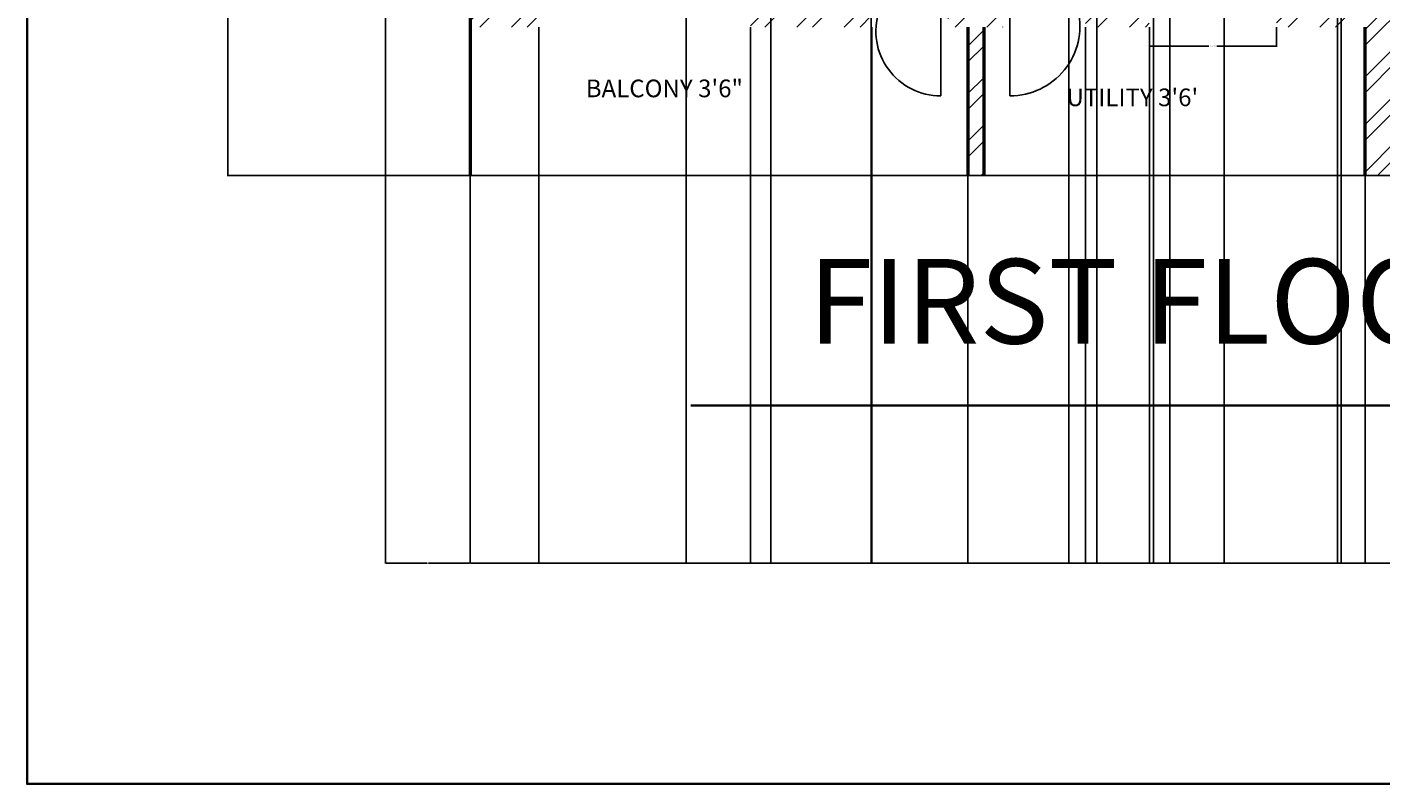
# Model space of a CAD drawing. Units: inches. Extents: x 1980 to 2738, y 1471 to 2568.
# Tile 1 of 22: x 1980 to 2363, y 1471 to 1686. Entities that reach past the tile are written whole.
import ezdxf

# ---------------------------------------------------------------- set-up
doc = ezdxf.new("R2010")
doc.units = ezdxf.units.IN
for name, color, linetype, lineweight in [('A-ANNO-DIMS', 2, 'Continuous', 18), ('A-ANNO-TTLB', 7, 'Continuous', 35), ('A-AREA-IDEN', 7, 'Continuous', 18), ('A-DOOR', 31, 'Continuous', 25), ('A-FLOR-BALC', 7, 'Continuous', 25), ('A-WALL', 7, 'Continuous', 50)]:
    doc.layers.add(name, color=color, linetype=linetype, lineweight=lineweight)
doc.layers.add('A-WALL-PATT', color=9, linetype='Continuous', lineweight=13, true_color=0xd19cc7)
doc.styles.get("Standard").update_dxf_attribs({"font": 'arial.ttf'})
doc.dimstyles.get("Standard").update_dxf_attribs({"dimtxt": 0.18, "dimasz": 0.18, "dimexe": 0.18, "dimexo": 0.0625, "dimgap": 0.09, "dimtad": 0, "dimtih": 1, "dimtoh": 1, "dimdec": 4, "dimzin": 0, "dimdsep": 46, "dimtxsty": 'Standard', "dimcen": 0.09, "dimadec": 0, "dimazin": 0, "dimtfac": 1, "dimtdec": 4, "dimtofl": 0, "dimtmove": 0, "dimatfit": 3, "dimfxl": 1, "dimtolj": 1, "dimtzin": 0, "dimarcsym": 0})

# ---------------------------------------------------------------- blocks, each defined once
blk = doc.blocks.new('*D31')
at = {"layer": 'A-ANNO-DIMS', "color": 0, "lineweight": -2, "transparency": 16777216}
for p, q in [((2297.48, 1685.64), (2297.48, 1680.13)), ((2333.48, 1685.64), (2333.48, 1680.13)), ((2297.66, 1680.31), (2314.36, 1680.31)), ((2333.3, 1680.31), (2316.59, 1680.31))]:
    blk.add_line(p, q, dxfattribs=at)
at = {"layer": 'A-ANNO-DIMS', "color": 0, "transparency": 16777216}
for points in [[(2297.66, 1680.34), (2297.66, 1680.28), (2297.48, 1680.31)], [(2333.3, 1680.34), (2333.3, 1680.28), (2333.48, 1680.31)]]:
    blk.add_solid(points, dxfattribs=at)
at = {"layer": 'Defpoints', "color": 0, "transparency": 16777216}
for p in [(2297.48, 1685.71), (2333.48, 1685.71), (2333.48, 1680.31)]:
    blk.add_point(p, dxfattribs=at)
at = {"layer": 'A-ANNO-DIMS', "color": 0, "transparency": 16777216, "insert": (2315.48, 1680.31), "char_height": 0.18, "attachment_point": 5}
blk.add_mtext('\\A1;WINDOW 36 TYP.', dxfattribs=at)
blk = doc.blocks.new('*D36')
at = {"layer": 'A-ANNO-DIMS', "color": 0, "lineweight": -2, "transparency": 16777216}
for p, q in [((2105.02, 2462.71), (2036.25, 2462.71)), ((2036.43, 2462.53), (2036.43, 2053.39)), ((2036.43, 1643.89), (2036.43, 2053.02)), ((2105.02, 1643.71), (2036.25, 1643.71))]:
    blk.add_line(p, q, dxfattribs=at)
at = {"layer": 'A-ANNO-DIMS', "color": 0, "transparency": 16777216}
for points in [[(2036.4, 2462.53), (2036.46, 2462.53), (2036.43, 2462.71)], [(2036.4, 1643.89), (2036.46, 1643.89), (2036.43, 1643.71)]]:
    blk.add_solid(points, dxfattribs=at)
at = {"layer": 'Defpoints', "color": 0, "transparency": 16777216}
for p in [(2036.43, 2462.71), (2105.08, 2462.71), (2105.08, 1643.71)]:
    blk.add_point(p, dxfattribs=at)
at = {"layer": 'A-ANNO-DIMS', "color": 0, "transparency": 16777216, "insert": (2036.43, 2053.21), "char_height": 0.18, "attachment_point": 5}
blk.add_mtext('\\A1;819', dxfattribs=at)
blk = doc.blocks.new('*D40')
at = {"layer": 'A-ANNO-DIMS', "color": 0, "lineweight": -2, "transparency": 16777216}
for p, q in [((2218.65, 2053.14), (2218.65, 1533.71)), ((2298.65, 2053.14), (2298.65, 1533.71)), ((2218.83, 1533.89), (2258.43, 1533.89)), ((2298.47, 1533.89), (2258.87, 1533.89))]:
    blk.add_line(p, q, dxfattribs=at)
at = {"layer": 'A-ANNO-DIMS', "color": 0, "transparency": 16777216}
for points in [[(2218.83, 1533.92), (2218.83, 1533.86), (2218.65, 1533.89)], [(2298.47, 1533.92), (2298.47, 1533.86), (2298.65, 1533.89)]]:
    blk.add_solid(points, dxfattribs=at)
at = {"layer": 'Defpoints', "color": 0, "transparency": 16777216}
for p in [(2218.65, 2053.21), (2298.65, 2053.21), (2298.65, 1533.89)]:
    blk.add_point(p, dxfattribs=at)
at = {"layer": 'A-ANNO-DIMS', "color": 0, "transparency": 16777216, "insert": (2258.65, 1533.89), "char_height": 0.18, "attachment_point": 5}
blk.add_mtext('\\A1;80', dxfattribs=at)
blk = doc.blocks.new('*D41')
at = {"layer": 'A-ANNO-DIMS', "color": 0, "lineweight": -2, "transparency": 16777216}
for p, q in [((2298.65, 2095.14), (2298.65, 1533.71)), ((2515.4, 2095.14), (2515.4, 1533.71)), ((2298.83, 1533.89), (2406.56, 1533.89)), ((2515.22, 1533.89), (2407.49, 1533.89))]:
    blk.add_line(p, q, dxfattribs=at)
at = {"layer": 'A-ANNO-DIMS', "color": 0, "transparency": 16777216}
for points in [[(2298.83, 1533.92), (2298.83, 1533.86), (2298.65, 1533.89)], [(2515.22, 1533.92), (2515.22, 1533.86), (2515.4, 1533.89)]]:
    blk.add_solid(points, dxfattribs=at)
at = {"layer": 'Defpoints', "color": 0, "transparency": 16777216}
for p in [(2298.65, 2095.21), (2515.4, 2095.21), (2515.4, 1533.89)]:
    blk.add_point(p, dxfattribs=at)
at = {"layer": 'A-ANNO-DIMS', "color": 0, "transparency": 16777216, "insert": (2407.03, 1533.89), "char_height": 0.18, "attachment_point": 5}
blk.add_mtext('\\A1;216.75', dxfattribs=at)
blk = doc.blocks.new('*D42')
at = {"layer": 'A-ANNO-DIMS', "color": 0, "lineweight": -2, "transparency": 16777216}
for p, q in [((2105.08, 1685.64), (2105.08, 1533.71)), ((2124.51, 1685.64), (2124.51, 1533.71)), ((2105.26, 1533.89), (2114.34, 1533.89)), ((2124.33, 1533.89), (2115.25, 1533.89))]:
    blk.add_line(p, q, dxfattribs=at)
at = {"layer": 'A-ANNO-DIMS', "color": 0, "transparency": 16777216}
for points in [[(2105.26, 1533.92), (2105.26, 1533.86), (2105.08, 1533.89)], [(2124.33, 1533.92), (2124.33, 1533.86), (2124.51, 1533.89)]]:
    blk.add_solid(points, dxfattribs=at)
at = {"layer": 'Defpoints', "color": 0, "transparency": 16777216}
for p in [(2105.08, 1685.71), (2124.51, 1685.71), (2124.51, 1533.89)]:
    blk.add_point(p, dxfattribs=at)
at = {"layer": 'A-ANNO-DIMS', "color": 0, "transparency": 16777216, "insert": (2114.8, 1533.89), "char_height": 0.18, "attachment_point": 5}
blk.add_mtext('\\A1;19.427', dxfattribs=at)
blk = doc.blocks.new('*D43')
at = {"layer": 'A-ANNO-DIMS', "color": 0, "lineweight": -2, "transparency": 16777216}
for p, q in [((2184.51, 1685.64), (2184.51, 1533.71)), ((2218.88, 1685.64), (2218.88, 1533.71)), ((2184.69, 1533.89), (2201.3, 1533.89)), ((2218.7, 1533.89), (2202.09, 1533.89))]:
    blk.add_line(p, q, dxfattribs=at)
at = {"layer": 'A-ANNO-DIMS', "color": 0, "transparency": 16777216}
for points in [[(2184.69, 1533.92), (2184.69, 1533.86), (2184.51, 1533.89)], [(2218.7, 1533.92), (2218.7, 1533.86), (2218.88, 1533.89)]]:
    blk.add_solid(points, dxfattribs=at)
at = {"layer": 'Defpoints', "color": 0, "transparency": 16777216}
for p in [(2184.51, 1685.71), (2218.88, 1685.71), (2218.88, 1533.89)]:
    blk.add_point(p, dxfattribs=at)
at = {"layer": 'A-ANNO-DIMS', "color": 0, "transparency": 16777216, "insert": (2201.69, 1533.89), "char_height": 0.18, "attachment_point": 5}
blk.add_mtext('\\A1;34.37', dxfattribs=at)
blk = doc.blocks.new('*D47')
at = {"layer": 'A-ANNO-DIMS', "color": 0, "lineweight": -2, "transparency": 16777216}
for p, q in [((2166.25, 1814.64), (2166.25, 1533.71)), ((2190.3, 1814.64), (2190.3, 1533.71)), ((2166.43, 1533.89), (2177.81, 1533.89)), ((2190.12, 1533.89), (2178.74, 1533.89))]:
    blk.add_line(p, q, dxfattribs=at)
at = {"layer": 'A-ANNO-DIMS', "color": 0, "transparency": 16777216}
for points in [[(2166.43, 1533.92), (2166.43, 1533.86), (2166.25, 1533.89)], [(2190.12, 1533.92), (2190.12, 1533.86), (2190.3, 1533.89)]]:
    blk.add_solid(points, dxfattribs=at)
at = {"layer": 'Defpoints', "color": 0, "transparency": 16777216}
for p in [(2166.25, 1814.71), (2190.3, 1814.71), (2190.3, 1533.89)]:
    blk.add_point(p, dxfattribs=at)
at = {"layer": 'A-ANNO-DIMS', "color": 0, "transparency": 16777216, "insert": (2178.28, 1533.89), "char_height": 0.18, "attachment_point": 5}
blk.add_mtext('\\A1;24.044', dxfattribs=at)
blk = doc.blocks.new('*D48')
at = {"layer": 'A-ANNO-DIMS', "color": 0, "lineweight": -2, "transparency": 16777216}
for p, q in [((2081.08, 1873.14), (2081.08, 1533.71)), ((2105.08, 1873.14), (2105.08, 1533.71)), ((2081.26, 1533.89), (2092.86, 1533.89)), ((2104.9, 1533.89), (2093.3, 1533.89))]:
    blk.add_line(p, q, dxfattribs=at)
at = {"layer": 'A-ANNO-DIMS', "color": 0, "transparency": 16777216}
for points in [[(2081.26, 1533.92), (2081.26, 1533.86), (2081.08, 1533.89)], [(2104.9, 1533.92), (2104.9, 1533.86), (2105.08, 1533.89)]]:
    blk.add_solid(points, dxfattribs=at)
at = {"layer": 'Defpoints', "color": 0, "transparency": 16777216}
for p in [(2081.08, 1873.21), (2105.08, 1873.21), (2105.08, 1533.89)]:
    blk.add_point(p, dxfattribs=at)
at = {"layer": 'A-ANNO-DIMS', "color": 0, "transparency": 16777216, "insert": (2093.08, 1533.89), "char_height": 0.18, "attachment_point": 5}
blk.add_mtext('\\A1;24', dxfattribs=at)
blk = doc.blocks.new('*D53')
at = {"layer": 'A-ANNO-DIMS', "color": 0, "lineweight": -2, "transparency": 16777216}
for p, q in [((2318.63, 2002.14), (2318.63, 1533.71)), ((2350.79, 2002.14), (2350.79, 1533.71)), ((2318.81, 1533.89), (2334.25, 1533.89)), ((2350.61, 1533.89), (2335.18, 1533.89))]:
    blk.add_line(p, q, dxfattribs=at)
at = {"layer": 'A-ANNO-DIMS', "color": 0, "transparency": 16777216}
for points in [[(2318.81, 1533.92), (2318.81, 1533.86), (2318.63, 1533.89)], [(2350.61, 1533.92), (2350.61, 1533.86), (2350.79, 1533.89)]]:
    blk.add_solid(points, dxfattribs=at)
at = {"layer": 'Defpoints', "color": 0, "transparency": 16777216}
for p in [(2318.63, 2002.21), (2350.79, 2002.21), (2350.79, 1533.89)]:
    blk.add_point(p, dxfattribs=at)
at = {"layer": 'A-ANNO-DIMS', "color": 0, "transparency": 16777216, "insert": (2334.71, 1533.89), "char_height": 0.18, "attachment_point": 5}
blk.add_mtext('\\A1;32.155', dxfattribs=at)
blk = doc.blocks.new('*D57')
at = {"layer": 'A-ANNO-DIMS', "color": 0, "lineweight": -2, "transparency": 16777216}
for p, q in [((2351.81, 1792.14), (2351.81, 1533.71)), ((2372.53, 1792.14), (2372.53, 1533.71)), ((2351.99, 1533.89), (2361.77, 1533.89)), ((2372.35, 1533.89), (2362.56, 1533.89))]:
    blk.add_line(p, q, dxfattribs=at)
at = {"layer": 'A-ANNO-DIMS', "color": 0, "transparency": 16777216}
for points in [[(2351.99, 1533.92), (2351.99, 1533.86), (2351.81, 1533.89)], [(2372.35, 1533.92), (2372.35, 1533.86), (2372.53, 1533.89)]]:
    blk.add_solid(points, dxfattribs=at)
at = {"layer": 'Defpoints', "color": 0, "transparency": 16777216}
for p in [(2351.81, 1792.21), (2372.53, 1792.21), (2372.53, 1533.89)]:
    blk.add_point(p, dxfattribs=at)
at = {"layer": 'A-ANNO-DIMS', "color": 0, "transparency": 16777216, "insert": (2362.17, 1533.89), "char_height": 0.18, "attachment_point": 5}
blk.add_mtext('\\A1;20.72', dxfattribs=at)
blk = doc.blocks.new('*D59')
at = {"layer": 'A-ANNO-DIMS', "color": 0, "lineweight": -2, "transparency": 16777216}
for p, q in [((2105.08, 1643.64), (2105.08, 1533.71)), ((2246.08, 1643.64), (2246.08, 1533.71)), ((2105.26, 1533.89), (2175.32, 1533.89)), ((2245.9, 1533.89), (2175.85, 1533.89))]:
    blk.add_line(p, q, dxfattribs=at)
at = {"layer": 'A-ANNO-DIMS', "color": 0, "transparency": 16777216}
for points in [[(2105.26, 1533.92), (2105.26, 1533.86), (2105.08, 1533.89)], [(2245.9, 1533.92), (2245.9, 1533.86), (2246.08, 1533.89)]]:
    blk.add_solid(points, dxfattribs=at)
at = {"layer": 'Defpoints', "color": 0, "transparency": 16777216}
for p in [(2105.08, 1643.71), (2246.08, 1643.71), (2246.08, 1533.89)]:
    blk.add_point(p, dxfattribs=at)
at = {"layer": 'A-ANNO-DIMS', "color": 0, "transparency": 16777216, "insert": (2175.58, 1533.89), "char_height": 0.18, "attachment_point": 5}
blk.add_mtext('\\A1;141', dxfattribs=at)
blk = doc.blocks.new('*D60')
at = {"layer": 'A-ANNO-DIMS', "color": 0, "lineweight": -2, "transparency": 16777216}
for p, q in [((2246.08, 1643.64), (2246.08, 1533.71)), ((2358.58, 1643.64), (2358.58, 1533.71)), ((2246.26, 1533.89), (2301.95, 1533.89)), ((2358.4, 1533.89), (2302.72, 1533.89))]:
    blk.add_line(p, q, dxfattribs=at)
at = {"layer": 'A-ANNO-DIMS', "color": 0, "transparency": 16777216}
for points in [[(2246.26, 1533.92), (2246.26, 1533.86), (2246.08, 1533.89)], [(2358.4, 1533.92), (2358.4, 1533.86), (2358.58, 1533.89)]]:
    blk.add_solid(points, dxfattribs=at)
at = {"layer": 'Defpoints', "color": 0, "transparency": 16777216}
for p in [(2246.08, 1643.71), (2358.58, 1643.71), (2358.58, 1533.89)]:
    blk.add_point(p, dxfattribs=at)
at = {"layer": 'A-ANNO-DIMS', "color": 0, "transparency": 16777216, "insert": (2302.33, 1533.89), "char_height": 0.18, "attachment_point": 5}
blk.add_mtext('\\A1;112.5', dxfattribs=at)
blk = doc.blocks.new('*D63')
at = {"layer": 'A-ANNO-DIMS', "color": 0, "lineweight": -2, "transparency": 16777216}
for p, q in [((2279.39, 1685.64), (2279.39, 1533.71)), ((2297.48, 1685.64), (2297.48, 1533.71)), ((2279.57, 1533.89), (2287.98, 1533.89)), ((2297.3, 1533.89), (2288.89, 1533.89))]:
    blk.add_line(p, q, dxfattribs=at)
at = {"layer": 'A-ANNO-DIMS', "color": 0, "transparency": 16777216}
for points in [[(2279.57, 1533.92), (2279.57, 1533.86), (2279.39, 1533.89)], [(2297.3, 1533.92), (2297.3, 1533.86), (2297.48, 1533.89)]]:
    blk.add_solid(points, dxfattribs=at)
at = {"layer": 'Defpoints', "color": 0, "transparency": 16777216}
for p in [(2279.39, 1685.71), (2297.48, 1685.71), (2297.48, 1533.89)]:
    blk.add_point(p, dxfattribs=at)
at = {"layer": 'A-ANNO-DIMS', "color": 0, "transparency": 16777216, "insert": (2288.43, 1533.89), "char_height": 0.18, "attachment_point": 5}
blk.add_mtext('\\A1;18.083', dxfattribs=at)
blk = doc.blocks.new('*D64')
at = {"layer": 'A-ANNO-DIMS', "color": 0, "lineweight": -2, "transparency": 16777216}
for p, q in [((2303.33, 2002.14), (2303.33, 1533.71)), ((2318.63, 2002.14), (2318.63, 1533.71)), ((2303.51, 1533.89), (2310.67, 1533.89)), ((2318.45, 1533.89), (2311.3, 1533.89))]:
    blk.add_line(p, q, dxfattribs=at)
at = {"layer": 'A-ANNO-DIMS', "color": 0, "transparency": 16777216}
for points in [[(2303.51, 1533.92), (2303.51, 1533.86), (2303.33, 1533.89)], [(2318.45, 1533.92), (2318.45, 1533.86), (2318.63, 1533.89)]]:
    blk.add_solid(points, dxfattribs=at)
at = {"layer": 'Defpoints', "color": 0, "transparency": 16777216}
for p in [(2303.33, 2002.21), (2318.63, 2002.21), (2318.63, 1533.89)]:
    blk.add_point(p, dxfattribs=at)
at = {"layer": 'A-ANNO-DIMS', "color": 0, "transparency": 16777216, "insert": (2310.98, 1533.89), "char_height": 0.18, "attachment_point": 5}
blk.add_mtext('\\A1;15.3', dxfattribs=at)
blk = doc.blocks.new('*D66')
at = {"layer": 'A-ANNO-DIMS', "color": 0, "lineweight": -2, "transparency": 16777216}
for p, q in [((2274.65, 2095.14), (2274.65, 1533.71)), ((2282.65, 2095.14), (2282.65, 1533.71)), ((2274.83, 1533.89), (2278.5, 1533.89)), ((2282.47, 1533.89), (2278.8, 1533.89))]:
    blk.add_line(p, q, dxfattribs=at)
at = {"layer": 'A-ANNO-DIMS', "color": 0, "transparency": 16777216}
for points in [[(2274.83, 1533.92), (2274.83, 1533.86), (2274.65, 1533.89)], [(2282.47, 1533.92), (2282.47, 1533.86), (2282.65, 1533.89)]]:
    blk.add_solid(points, dxfattribs=at)
at = {"layer": 'Defpoints', "color": 0, "transparency": 16777216}
for p in [(2274.65, 2095.21), (2282.65, 2095.21), (2282.65, 1533.89)]:
    blk.add_point(p, dxfattribs=at)
at = {"layer": 'A-ANNO-DIMS', "color": 0, "transparency": 16777216, "insert": (2278.65, 1533.89), "char_height": 0.18, "attachment_point": 5}
blk.add_mtext('\\A1;8', dxfattribs=at)

msp = doc.modelspace()

# ---------------------------------------------------------------- hatches: boundary and pattern name
at = {"layer": 'A-WALL-PATT'}
h = msp.add_hatch(dxfattribs=at)
h.set_pattern_fill('ANSI32', color=256)
h.paths.add_polyline_path([(2257.5661, 2416.2064), (2257.5661, 2420.7064), (2250.5833, 2420.7064), (2250.5833, 2462.7064), (2246.0833, 2462.7064), (2246.0833, 2420.7064), (2237.0791, 2420.7064), (2237.0791, 2411.7064), (2246.0833, 2411.7064), (2246.0833, 2291.7064), (2242.6109, 2291.7064), (2242.6109, 2287.2064), (2246.0833, 2287.2064), (2250.5833, 2287.2064), (2250.5833, 2291.7064), (2250.5833, 2411.7064), (2257.5661, 2411.7064)])
h.paths.add_polyline_path([(2387.0396, 2416.2064), (2387.0396, 2420.7064), (2367.5833, 2420.7064), (2367.5833, 2462.7064), (2358.5833, 2462.7064), (2358.5833, 2420.7064), (2329.3087, 2420.7064), (2329.3087, 2411.7064), (2358.5833, 2411.7064), (2358.5833, 2321.7275), (2358.5833, 2309.7064), (2347.3089, 2309.7064), (2293.3089, 2309.7064), (2293.3089, 2259.0771), (2297.8089, 2259.0771), (2297.8089, 2305.2064), (2347.3089, 2305.2064), (2347.3089, 2284.7412), (2351.8089, 2284.7412), (2351.8089, 2305.2064), (2372.3188, 2305.2064), (2372.3761, 2284.3899), (2377.0295, 2284.3899), (2377.0295, 2299.3058), (2377.0295, 2305.2064), (2426.5295, 2305.2064), (2426.5295, 2257.5573), (2431.0295, 2257.5573), (2431.0295, 2309.7064), (2377.0295, 2309.7064), (2367.5833, 2309.7064), (2367.5833, 2321.7275), (2367.5833, 2411.7064), (2387.0396, 2411.7064)])
h.paths.add_polyline_path([(2448.5267, 2416.2064), (2448.5267, 2420.7064), (2423.0396, 2420.7064), (2423.0396, 2411.7064), (2448.5267, 2411.7064)])
h.paths.add_polyline_path([(2130.9128, 2416.2064), (2130.9128, 2420.7064), (2105.0833, 2420.7064), (2105.0833, 2386.6942), (2114.0833, 2386.6942), (2114.0833, 2411.7064), (2130.9128, 2411.7064)])
h.paths.add_polyline_path([(2212.9478, 2420.7064), (2190.9128, 2420.7064), (2190.9128, 2411.7064), (2212.9478, 2411.7064), (2212.9478, 2416.2064)])
h.paths.add_polyline_path([(2114.0833, 2326.6942), (2105.0833, 2326.6942), (2105.0833, 2291.7064), (2081.0833, 2291.7064), (2081.0833, 2287.2064), (2105.0833, 2287.2064), (2105.0833, 2276.1935), (2114.0833, 2276.1935), (2114.0833, 2287.2064), (2166.3825, 2287.2064), (2166.3825, 2289.4564), (2166.3825, 2291.7064), (2114.0833, 2291.7064)])
h.paths.add_polyline_path([(2114.0833, 2252.1935), (2105.0833, 2252.1935), (2105.0833, 2233.2064), (2081.0833, 2233.2064), (2081.0833, 2228.7064), (2105.0833, 2228.7064), (2105.0833, 2213.4478), (2114.0833, 2213.4478), (2114.0833, 2228.7064), (2195.0833, 2228.7064), (2199.5833, 2228.7064), (2208.4455, 2228.7064), (2208.4455, 2230.9564), (2208.4455, 2233.2064), (2199.5833, 2233.2064), (2199.5833, 2287.2064), (2206.8904, 2287.2064), (2206.8904, 2289.4564), (2206.8904, 2291.7064), (2189.446, 2291.7064), (2189.446, 2289.4564), (2189.446, 2287.2064), (2195.0833, 2287.2064), (2195.0833, 2233.2064), (2114.0833, 2233.2064)])
h.paths.add_polyline_path([(2114.0833, 2153.4478), (2109.5833, 2153.4478), (2105.0833, 2153.4478), (2105.0833, 2135.2374), (2114.0833, 2135.2374)], flags=17)
h.paths.add_polyline_path([(2135.9619, 2095.4081), (2140.1805, 2095.4081), (2140.1805, 2104.2064), (2114.0833, 2104.2064), (2114.0833, 2110.3997), (2109.5833, 2110.3997), (2105.0833, 2110.3997), (2105.0833, 2104.2064), (2081.0833, 2104.2064), (2081.0833, 2099.7064), (2105.0833, 2099.7064), (2127.5416, 2099.8532), (2127.5416, 2056.9393), (2136.2133, 2056.9393)], flags=17)
h.paths.add_polyline_path([(2255.4895, 2104.2064), (2250.5833, 2104.2064), (2250.5833, 2233.2064), (2246.0833, 2233.2064), (2242.4941, 2233.2064), (2242.4941, 2228.7064), (2246.0833, 2228.7064), (2246.0833, 2104.2064), (2163.6825, 2104.2064), (2163.6825, 2099.8072), (2163.6825, 2095.4081), (2191.4325, 2095.4081), (2191.4325, 2011.2064), (2186.0833, 2011.2064), (2136.5143, 2010.8824), (2136.3702, 2032.9403), (2131.9559, 2032.9115), (2127.5416, 2032.8826), (2127.5416, 2006.7064), (2105.0833, 2006.7064), (2081.0833, 2006.7064), (2081.0833, 2002.2064), (2105.0833, 2002.2064), (2105.0833, 1995.9329), (2114.0833, 1995.9329), (2114.0833, 2002.2064), (2246.0833, 2002.2064), (2246.0833, 1877.7064), (2242.1358, 1877.7064), (2242.1358, 1873.2064), (2250.5833, 1873.2064), (2250.5833, 2002.2064), (2255.3335, 2002.2064), (2255.3335, 2011.2064), (2195.9325, 2011.2064), (2195.9325, 2095.2064), (2255.4895, 2095.2064), (2255.4895, 2099.5471)])
h.paths.add_polyline_path([(2199.5833, 1873.2064), (2209.827, 1873.2064), (2209.827, 1875.4564), (2209.827, 1877.7064), (2114.0833, 1877.7064), (2114.0833, 1890.0968), (2105.0833, 1890.0968), (2105.0833, 1877.7064), (2081.0833, 1877.7064), (2081.0833, 1873.2064), (2105.0833, 1873.2064), (2105.0833, 1857.7279), (2114.0833, 1857.7279), (2114.0833, 1873.2064), (2195.0833, 1873.2064), (2195.0833, 1819.2064), (2190.298, 1819.2064), (2190.298, 1814.7064), (2209.8976, 1814.7064), (2209.8976, 1816.9564), (2209.8976, 1819.2064), (2199.5833, 1819.2064)])
h.paths.add_polyline_path([(2114.0833, 1814.7064), (2166.2538, 1814.7064), (2166.2538, 1816.9564), (2166.2538, 1819.2064), (2114.0833, 1819.2064), (2114.0833, 1833.7279), (2109.5833, 1833.7279), (2105.0833, 1833.7279), (2105.0833, 1819.2064), (2081.0833, 1819.2064), (2081.0833, 1814.7064), (2105.0833, 1814.7064), (2105.0833, 1782.5516), (2114.0833, 1782.5516)])
h.paths.add_polyline_path([(2114.0833, 1722.5516), (2109.5833, 1722.5516), (2105.0833, 1722.5516), (2105.0833, 1685.7064), (2124.5104, 1685.7064), (2124.5104, 1690.2064), (2124.5104, 1694.7064), (2114.0833, 1694.7064)])
h.paths.add_polyline_path([(2218.8787, 1694.7064), (2184.5104, 1694.7064), (2184.5104, 1685.7064), (2218.8787, 1685.7064), (2218.8787, 1690.2064)])
h.paths.add_polyline_path([(2250.5833, 1819.2064), (2242.6431, 1819.2064), (2242.6431, 1816.9564), (2242.6431, 1814.7064), (2246.0833, 1814.7064), (2246.0833, 1694.7064), (2240.4035, 1694.7064), (2240.4035, 1690.2064), (2240.4035, 1685.7064), (2246.0833, 1685.7064), (2246.0833, 1643.7064), (2250.5833, 1643.7064), (2250.5833, 1685.7064), (2255.9859, 1685.7064), (2255.9859, 1690.2064), (2255.9859, 1694.7064), (2250.5833, 1694.7064)])
h.paths.add_polyline_path([(2297.4764, 1694.7064), (2279.3934, 1694.7064), (2279.3934, 1690.2064), (2279.3934, 1685.7064), (2297.4764, 1685.7064), (2297.4764, 1690.2064)])
h.paths.add_polyline_path([(2377.1596, 1694.7064), (2367.5833, 1694.7064), (2367.5833, 1787.7064), (2431.0295, 1787.7064), (2431.0295, 1792.2064), (2431.0295, 1849.4149), (2428.7795, 1849.4149), (2426.5295, 1849.4149), (2426.5295, 1792.2064), (2421.5833, 1792.2064), (2367.5833, 1792.2064), (2297.8089, 1792.2064), (2297.8089, 1850.2946), (2295.5589, 1850.2946), (2293.3089, 1850.2946), (2293.3089, 1792.2064), (2293.3089, 1787.7064), (2297.8089, 1787.7064), (2358.5833, 1787.7064), (2358.5833, 1694.7064), (2333.4764, 1694.7064), (2333.4764, 1685.7064), (2358.5833, 1685.7064), (2358.5833, 1643.7064), (2367.5833, 1643.7064), (2367.5833, 1685.7064), (2377.1596, 1685.7064)])
h.paths.add_polyline_path([(2442.4912, 1694.7064), (2413.1596, 1694.7064), (2413.1596, 1685.7064), (2442.4912, 1685.7064)])
h.paths.add_polyline_path([(2480.0833, 1814.7064), (2483.4816, 1814.7064), (2483.4816, 1817.9384), (2483.4816, 1819.2064), (2475.5833, 1819.2064), (2475.5833, 1694.7064), (2470.7283, 1694.7064), (2470.7283, 1685.7064), (2475.5833, 1685.7064), (2475.5833, 1643.7064), (2480.0833, 1643.7064), (2480.0833, 1685.7064), (2486.3293, 1685.7064), (2486.3293, 1690.2064), (2486.3293, 1694.7064), (2480.0833, 1694.7064)])
h.paths.add_polyline_path([(2621.0833, 1721.7349), (2612.0833, 1721.7349), (2612.0833, 1694.7064), (2586.1453, 1694.7064), (2586.1453, 1685.7064), (2621.0833, 1685.7064)])
h.paths.add_polyline_path([(2526.1453, 1690.2064), (2526.1453, 1694.7064), (2511.584, 1694.7064), (2511.584, 1690.2064), (2511.584, 1685.7064), (2526.1453, 1685.7064)])
h.paths.add_polyline_path([(2645.0833, 1819.2064), (2621.0833, 1819.2064), (2621.0833, 1835.8527), (2616.5833, 1835.8527), (2612.0833, 1835.8527), (2612.0833, 1819.2064), (2560.2541, 1819.2064), (2560.2541, 1814.7064), (2612.0833, 1814.7064), (2612.0833, 1781.7349), (2621.0833, 1781.7349), (2621.0833, 1814.7064), (2645.0833, 1814.7064)])
h.paths.add_polyline_path([(2645.0833, 1877.7064), (2621.0833, 1877.7064), (2621.0833, 1886.4375), (2612.0833, 1886.4375), (2612.0833, 1877.7064), (2517.1032, 1877.7064), (2517.1032, 1875.4564), (2517.1032, 1873.2064), (2526.5833, 1873.2064), (2526.5833, 1819.2064), (2516.6454, 1819.2064), (2516.6454, 1816.9564), (2516.6454, 1814.7064), (2536.4445, 1814.7064), (2536.4445, 1816.9564), (2536.4445, 1819.2064), (2531.0833, 1819.2064), (2531.0833, 1873.2064), (2612.0833, 1873.2064), (2612.0833, 1859.8527), (2621.0833, 1859.8527), (2621.0833, 1873.2064), (2645.0833, 1873.2064)])
h.paths.add_polyline_path([(2645.0833, 2006.7064), (2621.0833, 2006.7064), (2588.5085, 2006.7064), (2588.5085, 2052.9125), (2579.9045, 2052.9125), (2579.9045, 2011.2064), (2519.9045, 2011.2064), (2519.9045, 2095.2064), (2553.1204, 2095.2064), (2553.1204, 2104.2064), (2480.0833, 2104.2064), (2480.0833, 2228.7064), (2484.3832, 2228.7064), (2484.3832, 2230.9564), (2484.3832, 2233.2064), (2475.5833, 2233.2064), (2475.5833, 2104.2064), (2463.1308, 2104.2064), (2463.1308, 2095.2064), (2501.2463, 2095.2064), (2510.9045, 2095.2064), (2515.4045, 2095.2064), (2515.4045, 2011.2064), (2510.9045, 2011.2064), (2501.2463, 2011.2064), (2462.5957, 2011.2064), (2462.5957, 2002.2064), (2475.5833, 2002.2064), (2475.5833, 1873.2064), (2483.6146, 1873.2064), (2483.6146, 1875.4564), (2483.6146, 1877.7064), (2480.0833, 1877.7064), (2480.0833, 2002.2064), (2612.0833, 2002.2064), (2612.0833, 1996.309), (2621.0833, 1996.309), (2621.0833, 2002.2064), (2645.0833, 2002.2064)])
h.paths.add_polyline_path([(2588.5085, 2099.7277), (2621.0833, 2099.7277), (2645.0833, 2099.7064), (2645.0833, 2104.2064), (2621.0833, 2104.2064), (2621.0833, 2109.0038), (2616.5833, 2109.0038), (2612.0833, 2109.0038), (2612.0833, 2104.2064), (2575.0621, 2104.2064), (2575.0621, 2099.7064), (2575.0621, 2095.2064), (2579.9045, 2095.2064), (2579.9045, 2076.9125), (2588.5085, 2076.9125)], flags=17)
h.paths.add_polyline_path([(2367.5833, 2002.2064), (2373.7228, 2002.2064), (2373.7228, 2006.7064), (2373.7228, 2011.2064), (2350.7889, 2011.2064), (2350.7889, 2006.7064), (2350.7889, 2002.2064), (2358.5833, 2002.2064), (2358.5833, 1877.7064), (2293.3089, 1877.7064), (2293.3089, 1870.4987), (2297.8089, 1870.4987), (2297.8089, 1873.2064), (2347.3089, 1873.2064), (2347.3089, 1847.2208), (2351.8089, 1847.2208), (2351.8089, 1873.2064), (2372.5295, 1873.2064), (2372.5295, 1847.8619), (2377.0295, 1847.8619), (2377.0295, 1873.2064), (2426.5295, 1873.2064), (2426.5295, 1868.7339), (2431.0295, 1868.7339), (2431.0295, 1877.7064), (2367.5833, 1877.7064)])
h.paths.add_polyline_path([(2531.0833, 2287.2064), (2534.2285, 2287.2064), (2534.2285, 2291.7064), (2516.7886, 2291.7064), (2516.7886, 2287.2064), (2526.5833, 2287.2064), (2526.5833, 2233.2064), (2517.9112, 2233.2064), (2517.9112, 2230.9564), (2517.9112, 2228.7064), (2526.5833, 2228.7064), (2531.0833, 2228.7064), (2612.0833, 2228.7064), (2612.0833, 2206.8504), (2621.0833, 2206.8504), (2621.0833, 2228.7064), (2645.0833, 2228.7064), (2645.0833, 2233.2064), (2621.0833, 2233.2064), (2621.0833, 2241.8536), (2616.5833, 2241.8536), (2612.0833, 2241.8536), (2612.0833, 2233.2064), (2531.0833, 2233.2064)])
h.paths.add_polyline_path([(2645.0833, 2291.7064), (2621.0833, 2291.7064), (2621.0833, 2323.0138), (2616.5833, 2323.0138), (2612.0833, 2323.0138), (2612.0833, 2291.7064), (2559.6852, 2291.7064), (2559.6852, 2289.4564), (2559.6852, 2287.2064), (2612.0833, 2287.2064), (2612.0833, 2265.8536), (2621.0833, 2265.8536), (2621.0833, 2287.2064), (2645.0833, 2287.2064)])
h.paths.add_polyline_path([(2621.0833, 2420.7064), (2582.8189, 2420.7064), (2582.8189, 2411.7064), (2612.0833, 2411.7064), (2612.0833, 2383.0138), (2621.0833, 2383.0138)])
h.paths.add_polyline_path([(2480.0833, 2411.7064), (2485.7342, 2411.7064), (2485.7342, 2416.2064), (2485.7342, 2420.7064), (2480.0833, 2420.7064), (2480.0833, 2462.7064), (2475.5833, 2462.7064), (2475.5833, 2420.7064), (2469.4083, 2420.7064), (2469.4083, 2411.7064), (2475.5833, 2411.7064), (2475.5833, 2291.7064), (2475.5833, 2287.2064), (2482.9195, 2287.2064), (2482.9195, 2289.4564), (2482.9195, 2291.7064), (2480.0833, 2291.7064)])
h.paths.add_polyline_path([(2367.5833, 2228.7064), (2431.0295, 2228.7064), (2431.0295, 2233.2064), (2431.0295, 2237.4203), (2428.7795, 2237.4203), (2426.5295, 2237.4203), (2426.5295, 2233.2064), (2377.0295, 2233.2064), (2377.0295, 2260.3837), (2372.4423, 2260.3837), (2372.517, 2233.2635), (2351.8089, 2233.2064), (2351.8089, 2260.7412), (2347.3089, 2260.7412), (2347.3089, 2233.2064), (2297.8089, 2233.2064), (2297.8089, 2236.9324), (2293.3089, 2236.9324), (2293.3089, 2228.7064), (2358.5833, 2228.7064), (2358.5833, 2104.2064), (2353.3665, 2104.2064), (2353.3665, 2095.2064), (2373.8869, 2095.2064), (2373.8869, 2099.7064), (2373.8869, 2104.2064), (2367.5833, 2104.2064)])
h.paths.add_polyline_path([(2321.2323, 2104.2064), (2303.4895, 2104.2064), (2303.4895, 2095.2064), (2321.2323, 2095.2064), (2321.2323, 2099.7064)], flags=0)
h.paths.add_polyline_path([(2415.1308, 2099.7064), (2415.1308, 2104.2064), (2404.81, 2104.2064), (2404.81, 2095.2064), (2415.1308, 2095.2064)], flags=17)
h.paths.add_polyline_path([(2318.6336, 2011.2064), (2303.3335, 2011.2064), (2303.3335, 2002.2064), (2318.6336, 2002.2064)], flags=0)
h.paths.add_polyline_path([(2414.5957, 2011.2064), (2406.2461, 2011.2064), (2406.2461, 2006.7064), (2406.2461, 2002.2064), (2414.5957, 2002.2064)], flags=17)

# ---------------------------------------------------------------- linework, layer by layer
at = {"layer": 'A-ANNO-TTLB'}
msp.add_line((2167.6271, 1578.5357), (2534.552, 1578.5357), dxfattribs=at)
msp.add_lwpolyline([(1979.5621, 2567.5568), (2738.2543, 2567.5568), (2738.2543, 1471.317), (1979.5621, 1471.317)], close=True, dxfattribs=at)
at = {"layer": 'A-DOOR'}
for p, q in [((2238.4035, 1690.2064), (2238.4035, 1666.2064)), ((2257.9859, 1690.2064), (2257.9859, 1666.2064))]:
    msp.add_line(p, q, dxfattribs=at)
for centre, radius, start, end in [((2238.4035, 1684.6047), 18.3983, 162.273895, 270), ((2257.9859, 1686.0533), 19.8469, 270, 12.078851)]:
    msp.add_arc(centre, radius, start, end, dxfattribs=at)
at = {"layer": 'A-FLOR-BALC'}
msp.add_line((2621.0833, 1643.7064), (2105.0833, 1643.7064), dxfattribs=at)
at = {"layer": 'A-WALL'}
for p, q in [((2105.0833, 1722.5516), (2105.0833, 1643.7064)), ((2246.0833, 1685.7064), (2246.0833, 1643.7064)), ((2250.5833, 1685.7064), (2250.5833, 1643.7064)), ((2358.5833, 1643.7064), (2358.5833, 1685.7064))]:
    msp.add_line(p, q, dxfattribs=at)

# ---------------------------------------------------------------- texts
at = {"layer": 'A-ANNO-TTLB', "insert": (2200.9148, 1620.0295), "char_height": 24, "attachment_point": 1}
msp.add_mtext_dynamic_manual_height_columns('FIRST FLOOR PLAN', width=445.461587, gutter_width=12.5, heights=[0], dxfattribs=at)
at = {"layer": 'A-AREA-IDEN', "char_height": 5, "attachment_point": 1}
for s, width, insert in [('BALCONY 3\'6"', 312.91929, (2137.8231, 1670.8316)), ("UTILITY 3'6'", 259.710351, (2274.0127, 1668.2988))]:
    msp.add_mtext_dynamic_manual_height_columns(s, width=width, gutter_width=12.5, heights=[0], dxfattribs=dict(at, insert=insert))

# ---------------------------------------------------------------- dimensions: what is measured, and where the dimension line sits
at = {"layer": 'A-ANNO-DIMS'}
dim = msp.add_linear_dim(base=(2036.4333, 2462.7064), p1=(2105.0833, 1643.7064), p2=(2105.0833, 2462.7064), angle=90, dimstyle='Standard', override={"dimdec": 0, "dimlfac": 1, "dimrnd": 0, "dimzin": 0, "dimdsep": 46, "dimlunit": 2}, dxfattribs=at)
dim.commit()
dim.dimension.update_dxf_attribs({"geometry": '*D36', "text_midpoint": (2036.4333, 2053.2064)})
for base, p1, p2, override, picture, middle in [((2282.6516, 1533.8857), (2274.6516, 2095.2064), (2282.6516, 2095.2064), {"dimdec": 0, "dimlfac": 1, "dimrnd": 0, "dimzin": 0, "dimdsep": 46, "dimlunit": 2}, '*D66', (2278.6516, 1533.8857)), ((2515.4045, 1533.8857), (2298.6516, 2095.2064), (2515.4045, 2095.2064), {"dimdec": 2, "dimlfac": 1, "dimrnd": 0, "dimzin": 0, "dimdsep": 46, "dimlunit": 2}, '*D41', (2407.0281, 1533.8857)), ((2298.6516, 1533.8857), (2218.6516, 2053.2064), (2298.6516, 2053.2064), {"dimdec": 0, "dimlfac": 1, "dimrnd": 0, "dimzin": 0, "dimdsep": 46, "dimlunit": 2}, '*D40', (2258.6516, 1533.8857)), ((2318.6336, 1533.8857), (2303.3335, 2002.2064), (2318.6336, 2002.2064), {"dimdec": 1, "dimlfac": 1, "dimrnd": 0, "dimzin": 0, "dimdsep": 46, "dimlunit": 2}, '*D64', (2310.9835, 1533.8857)), ((2350.7889, 1533.8857), (2318.6336, 2002.2064), (2350.7889, 2002.2064), {"dimdec": 3, "dimlfac": 1, "dimrnd": 0, "dimzin": 0, "dimdsep": 46, "dimlunit": 2}, '*D53', (2334.7112, 1533.8857)), ((2105.0833, 1533.8857), (2081.0833, 1873.2064), (2105.0833, 1873.2064), {"dimdec": 0, "dimlfac": 1, "dimrnd": 0, "dimzin": 0, "dimdsep": 46, "dimlunit": 2}, '*D48', (2093.0833, 1533.8857)), ((2190.298, 1533.8857), (2166.2538, 1814.7064), (2190.298, 1814.7064), {"dimdec": 3, "dimlfac": 1, "dimrnd": 0, "dimzin": 0, "dimdsep": 46, "dimlunit": 2}, '*D47', (2178.2759, 1533.8857)), ((2372.5295, 1533.8857), (2351.8089, 1792.2064), (2372.5295, 1792.2064), {"dimdec": 2, "dimlfac": 1, "dimrnd": 0, "dimzin": 0, "dimdsep": 46, "dimlunit": 2}, '*D57', (2362.1692, 1533.8857)), ((2124.5104, 1533.8857), (2105.0833, 1685.7064), (2124.5104, 1685.7064), {"dimdec": 3, "dimlfac": 1, "dimrnd": 0, "dimzin": 0, "dimdsep": 46, "dimlunit": 2}, '*D42', (2114.7968, 1533.8857)), ((2218.8787, 1533.8857), (2184.5104, 1685.7064), (2218.8787, 1685.7064), {"dimdec": 2, "dimlfac": 1, "dimrnd": 0, "dimzin": 0, "dimdsep": 46, "dimlunit": 2}, '*D43', (2201.6945, 1533.8857)), ((2297.4764, 1533.8857), (2279.3934, 1685.7064), (2297.4764, 1685.7064), {"dimdec": 3, "dimlfac": 1, "dimrnd": 0, "dimzin": 0, "dimdsep": 46, "dimlunit": 2}, '*D63', (2288.4349, 1533.8857)), ((2246.0833, 1533.8857), (2105.0833, 1643.7064), (2246.0833, 1643.7064), {"dimdec": 0, "dimlfac": 1, "dimrnd": 0, "dimzin": 0, "dimdsep": 46, "dimlunit": 2}, '*D59', (2175.5833, 1533.8857)), ((2358.5833, 1533.8857), (2246.0833, 1643.7064), (2358.5833, 1643.7064), {"dimdec": 1, "dimlfac": 1, "dimrnd": 0, "dimzin": 0, "dimdsep": 46, "dimlunit": 2}, '*D60', (2302.3333, 1533.8857))]:
    dim = msp.add_linear_dim(base=base, p1=p1, p2=p2, dimstyle='Standard', override=override, dxfattribs=at)
    dim.commit()
    dim.dimension.update_dxf_attribs({"geometry": picture, "text_midpoint": middle})
dim = msp.add_linear_dim(base=(2333.4764, 1680.3064), p1=(2297.4764, 1685.7064), p2=(2333.4764, 1685.7064), text='WINDOW <> TYP.', dimstyle='Standard', override={"dimdec": 0, "dimlfac": 1, "dimrnd": 0, "dimzin": 0, "dimdsep": 46, "dimlunit": 2}, dxfattribs=at)
dim.commit()
dim.dimension.update_dxf_attribs({"geometry": '*D31', "text_midpoint": (2315.4764, 1680.3064)})

doc.saveas('drawing.dxf')
